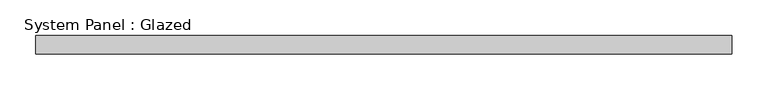
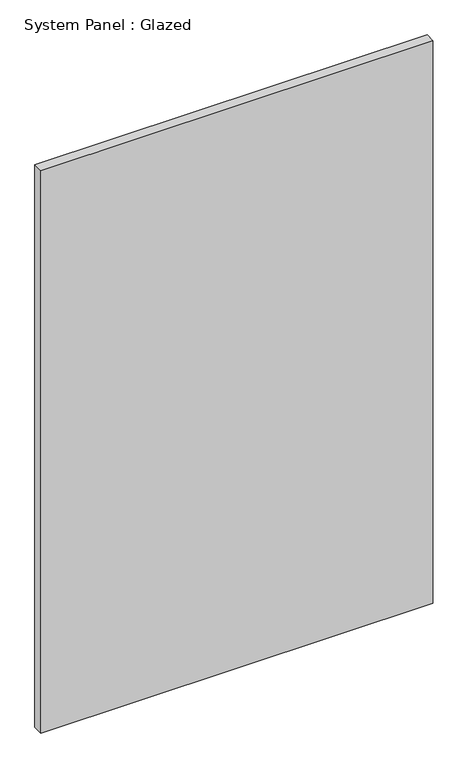
"""IFC4 building model written with IfcOpenShell, lengths in millimetres: plate geometry, System Panel : Glazed."""

from ifc_helpers import new_model, si_unit, origin, origin_with_axes, place, context, project, spatial, polyline, outline, extrude, source, transform, mapped, element, save


def system_panel_glazed_f5da27a7(model_context):
    return source(origin(), model_context, "Body", "SweptSolid", [
        extrude(outline(polyline([(485.775, 19.05), (-485.775, 19.05), (-485.775, 44.45), (485.775, 44.45), (485.775, 19.05)])), origin_with_axes(), (0.0, 0.0, 1.0), 1473.1465467),
    ])


if __name__ == "__main__":
    model = new_model("IFC4")
    model_context = context("Model", 3, world=origin())
    ifc_project = project(units=[si_unit("LENGTHUNIT", "METRE", prefix="MILLI")], contexts=[model_context])
    site = spatial("IfcSite", under=ifc_project)
    building = spatial("IfcBuilding", under=site)
    placement = place(None, origin())
    system_panel_glazed_shape = system_panel_glazed_f5da27a7(model_context)
    element("IfcPlate", 1, ObjectType="System Panel : Glazed", at=placement, inside=building, context=model_context, shape_type="MappedRepresentation", body=[
        mapped(system_panel_glazed_shape, transform((0.0, 0.0, 0.0), x_axis=(1.0, 0.0, 0.0), y_axis=(0.0, 1.0, 0.0), z_axis=(0.0, 0.0, 1.0))),
    ])
    save(model, "model.ifc")

# Revit data of these elements
# Type "System Panel : Glazed"
#   Construction Type Id = "GSP4R"
#   Analytic Construction = "1/8 in Pilkington single glazing"
#   Visual Light Transmittance = 0.9
#   Solar Heat Gain Coefficient = 0.86
#   Heat Transfer Coefficient (U) = 1.18115 BTU/(h·ft²·°F)
#   Define Thermal Properties by = 1
# Element 1 (IfcPlate, "System Panel : Glazed")
#   Materials on its faces: "Glass"
# Materials
#   "Glass": class "Glass", colour RGB 0 128 192, transparency 0.75, Description = "Soda Lime Glass", Cost = 0
